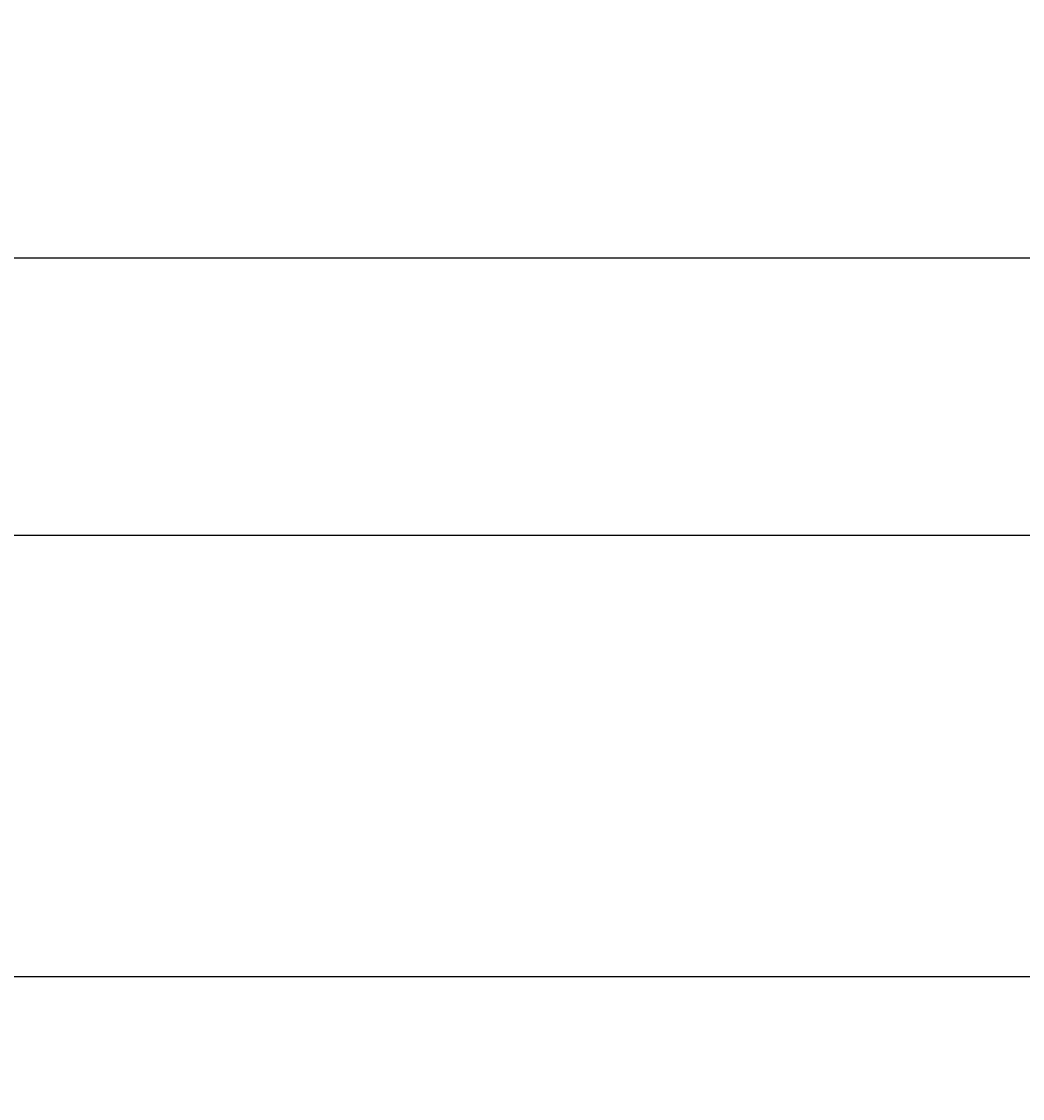
# Model space of a CAD drawing. Units: inches. Extents: x 35362 to 73946, y 43607 to 67532.
# Tile 16 of 134: x 46225 to 47763, y 45263 to 46919. Entities that reach past the tile are written whole.
import ezdxf

# ---------------------------------------------------------------- set-up
doc = ezdxf.new("R2010")
doc.units = ezdxf.units.IN
doc.header["$MEASUREMENT"] = 0
doc.layers.add('A-ANNO-DIMS', color=2, linetype='Continuous', lineweight=18)
doc.styles.get("Standard").update_dxf_attribs({"font": 'arial.ttf'})
doc.dimstyles.get("Standard").update_dxf_attribs({"dimtxt": 0.18, "dimasz": 0.18, "dimexe": 0.18, "dimexo": 0.0625, "dimgap": 0.09, "dimtad": 0, "dimtih": 1, "dimtoh": 1, "dimdec": 4, "dimzin": 0, "dimdsep": 46, "dimtxsty": 'Standard', "dimcen": 0.09, "dimadec": 0, "dimazin": 0, "dimtfac": 1, "dimtdec": 4, "dimtofl": 0, "dimtmove": 0, "dimatfit": 3, "dimfxl": 1, "dimtolj": 1, "dimtzin": 0, "dimarcsym": 0})

# ---------------------------------------------------------------- blocks, each defined once
blk = doc.blocks.new('*D5')
at = {"layer": 'A-ANNO-DIMS', "color": 0, "lineweight": -2, "transparency": 16777216}
for p, q in [((37121.9, 46919.3), (37121.9, 43606.7)), ((69871.5, 45449.8), (69871.5, 43606.7)), ((37122.1, 43606.9), (53496.3, 43606.9)), ((69871.3, 43606.9), (53497.2, 43606.9))]:
    blk.add_line(p, q, dxfattribs=at)
at = {"layer": 'A-ANNO-DIMS', "color": 0, "transparency": 16777216}
for points in [[(37122.1, 43606.9), (37122.1, 43606.8), (37121.9, 43606.9)], [(69871.3, 43606.9), (69871.3, 43606.8), (69871.5, 43606.9)]]:
    blk.add_solid(points, dxfattribs=at)
at = {"layer": 'Defpoints', "color": 0, "transparency": 16777216}
for p in [(37121.9, 46919.4), (69871.5, 45449.9), (69871.5, 43606.9)]:
    blk.add_point(p, dxfattribs=at)
at = {"layer": 'A-ANNO-DIMS', "color": 0, "transparency": 16777216, "insert": (53496.7, 43606.9), "char_height": 0.18, "attachment_point": 5}
blk.add_mtext('\\A1;32750', dxfattribs=at)
blk = doc.blocks.new('*D67')
at = {"layer": 'A-ANNO-DIMS', "color": 0, "lineweight": -2, "transparency": 16777216}
for p, q in [((56873.5, 53351.5), (35361.8, 53351.5)), ((35361.9, 53351.3), (35361.9, 49400.9)), ((35361.9, 45450.1), (35361.9, 49400.5)), ((53793.6, 45449.9), (35361.8, 45449.9))]:
    blk.add_line(p, q, dxfattribs=at)
at = {"layer": 'A-ANNO-DIMS', "color": 0, "transparency": 16777216}
for points in [[(35361.9, 53351.3), (35362, 53351.3), (35361.9, 53351.5)], [(35361.9, 45450.1), (35362, 45450.1), (35361.9, 45449.9)]]:
    blk.add_solid(points, dxfattribs=at)
at = {"layer": 'Defpoints', "color": 0, "transparency": 16777216}
for p in [(35361.9, 53351.5), (56873.6, 53351.5), (53793.6, 45449.9)]:
    blk.add_point(p, dxfattribs=at)
at = {"layer": 'A-ANNO-DIMS', "color": 0, "transparency": 16777216, "insert": (35361.9, 49400.7), "char_height": 0.18, "attachment_point": 5}
blk.add_mtext('\\A1;7901.6', dxfattribs=at)
blk = doc.blocks.new('*D76')
at = {"layer": 'A-ANNO-DIMS', "color": 0, "lineweight": -2, "transparency": 16777216}
for p, q in [((54052.8, 46555.3), (35361.8, 46555.3)), ((35361.9, 46555.1), (35361.9, 46342.3)), ((35361.9, 46129.1), (35361.9, 46341.9)), ((53793.6, 46128.9), (35361.8, 46128.9))]:
    blk.add_line(p, q, dxfattribs=at)
at = {"layer": 'A-ANNO-DIMS', "color": 0, "transparency": 16777216}
for points in [[(35361.9, 46555.1), (35362, 46555.1), (35361.9, 46555.3)], [(35361.9, 46129.1), (35362, 46129.1), (35361.9, 46128.9)]]:
    blk.add_solid(points, dxfattribs=at)
at = {"layer": 'Defpoints', "color": 0, "transparency": 16777216}
for p in [(35361.9, 46555.3), (54052.9, 46555.3), (53793.6, 46128.9)]:
    blk.add_point(p, dxfattribs=at)
at = {"layer": 'A-ANNO-DIMS', "color": 0, "transparency": 16777216, "insert": (35361.9, 46342.1), "char_height": 0.18, "attachment_point": 5}
blk.add_mtext('\\A1;426.4', dxfattribs=at)
blk = doc.blocks.new('*D90')
at = {"layer": 'A-ANNO-DIMS', "color": 0, "lineweight": -2, "transparency": 16777216}
for p, q in [((53707.7, 47291.3), (35361.8, 47291.3)), ((35361.9, 47291.1), (35361.9, 46710.3)), ((35361.9, 46129.1), (35361.9, 46709.9)), ((53793.6, 46128.9), (35361.8, 46128.9))]:
    blk.add_line(p, q, dxfattribs=at)
at = {"layer": 'A-ANNO-DIMS', "color": 0, "transparency": 16777216}
for points in [[(35361.9, 47291.1), (35362, 47291.1), (35361.9, 47291.3)], [(35361.9, 46129.1), (35362, 46129.1), (35361.9, 46128.9)]]:
    blk.add_solid(points, dxfattribs=at)
at = {"layer": 'Defpoints', "color": 0, "transparency": 16777216}
for p in [(53707.8, 47291.3), (35361.9, 46128.9), (53793.6, 46128.9)]:
    blk.add_point(p, dxfattribs=at)
at = {"layer": 'A-ANNO-DIMS', "color": 0, "transparency": 16777216, "insert": (35361.9, 46710.1), "char_height": 0.18, "attachment_point": 5}
blk.add_mtext('\\A1;1162.4', dxfattribs=at)

msp = doc.modelspace()

# ---------------------------------------------------------------- dimensions: what is measured, and where the dimension line sits
at = {"layer": 'A-ANNO-DIMS'}
for base, p1, p2, picture, middle in [((35361.949, 53351.529), (53793.638, 45449.894), (56873.602, 53351.529), '*D67', (35361.949, 49400.712)), ((35361.949, 46128.878), (53707.781, 47291.285), (53793.638, 46128.878), '*D90', (35361.949, 46710.081)), ((35361.949, 46555.293), (53793.638, 46128.878), (54052.899, 46555.293), '*D76', (35361.949, 46342.086))]:
    dim = msp.add_linear_dim(base=base, p1=p1, p2=p2, angle=90, dimstyle='Standard', override={"dimdec": 1, "dimlfac": 1, "dimrnd": 0, "dimzin": 0, "dimdsep": 46, "dimlunit": 2}, dxfattribs=at)
    dim.commit()
    dim.dimension.update_dxf_attribs({"geometry": picture, "text_midpoint": middle})
dim = msp.add_linear_dim(base=(69871.496, 43606.859), p1=(37121.949, 46919.381), p2=(69871.496, 45449.894), dimstyle='Standard', override={"dimdec": 0, "dimlfac": 1, "dimrnd": 0, "dimzin": 0, "dimdsep": 46, "dimlunit": 2}, dxfattribs=at)
dim.commit()
dim.dimension.update_dxf_attribs({"geometry": '*D5', "text_midpoint": (53496.723, 43606.859)})

doc.saveas('drawing.dxf')
